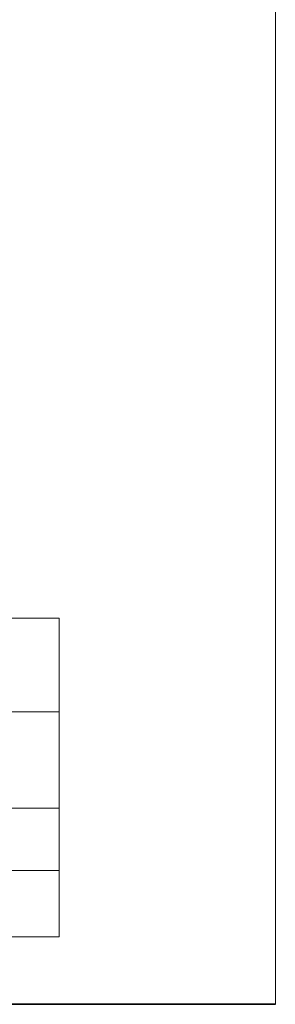
# Model space of a CAD drawing. Units: millimetres. Extents: x 20768 to 23556, y 50760 to 52704.
# Tile 32 of 36: x 22556 to 22720, y 50976 to 51606. Entities that reach past the tile are written whole.
import ezdxf

# ---------------------------------------------------------------- set-up
doc = ezdxf.new("R2010")
doc.units = ezdxf.units.MM
doc.layers.add('A-ANNO-SCHD', color=7, linetype='Continuous', lineweight=18)
doc.layers.add('A-ANNO-TTLB', color=7, linetype='Continuous', lineweight=35)

msp = doc.modelspace()

# ---------------------------------------------------------------- linework, layer by layer
at = {"layer": 'A-ANNO-SCHD'}
for p, q in [((22719.7, 51623.53), (22719.7, 50975.78)), ((21901.26, 51223.03), (22580.95, 51223.03)), ((22580.95, 51223.03), (22580.95, 51019.03)), ((21901.26, 51163.03), (22580.95, 51163.03)), ((21901.26, 51101.3), (22580.95, 51101.3)), ((21901.26, 51061.4), (22580.95, 51061.4)), ((21901.26, 51019.03), (22580.95, 51019.03))]:
    msp.add_line(p, q, dxfattribs=at)
at = {"layer": 'A-ANNO-TTLB'}
msp.add_line((20768.14, 50975.78), (22719.7, 50975.78), dxfattribs=at)

doc.saveas('drawing.dxf')
